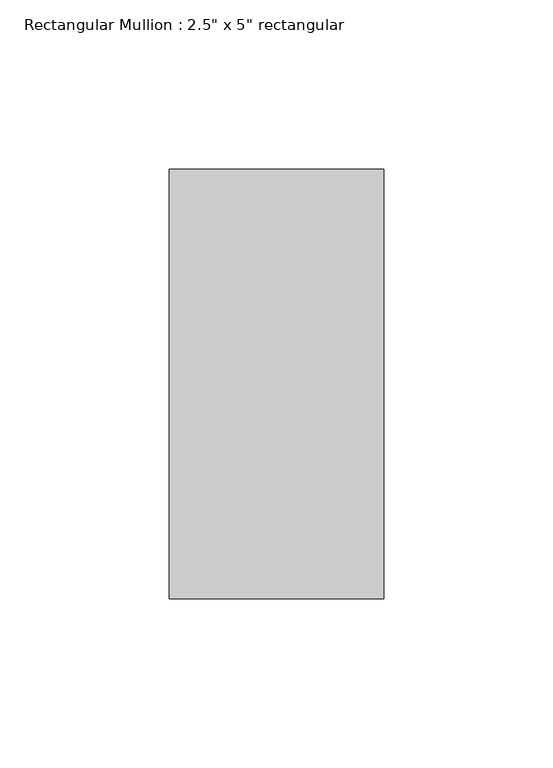
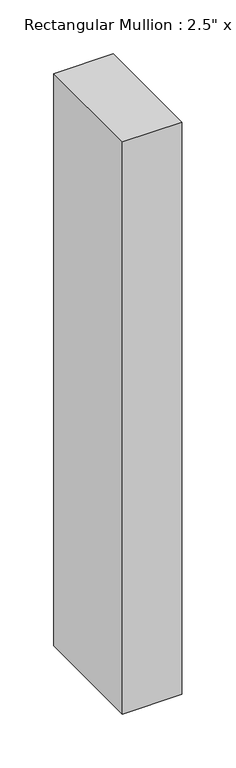
"""IFC4 building model written with IfcOpenShell, lengths in millimetres: member geometry."""

from ifc_helpers import new_model, si_unit, frame, origin, place, context, project, spatial, polyline, outline, extrude, source, transform, mapped, element, save


def member_5215b92c(model_context):
    return source(origin(), model_context, "Body", "SweptSolid", [
        extrude(outline(polyline([(0.0, 63.5), (0.0, -63.5), (-63.5, -63.5), (-63.5, 63.5), (0.0, 63.5)])), frame((0.0, 0.0, -647.7), z_axis=(0.0, 0.0, 1.0), x_axis=(1.0, 0.0, 0.0)), (0.0, 0.0, 1.0), 647.7),
    ])


if __name__ == "__main__":
    model = new_model("IFC4")
    model_context = context("Model", 3, world=origin())
    ifc_project = project(units=[si_unit("LENGTHUNIT", "METRE", prefix="MILLI")], contexts=[model_context])
    site = spatial("IfcSite", under=ifc_project)
    building = spatial("IfcBuilding", under=site)
    placement = place(None, origin())
    member_shape = member_5215b92c(model_context)
    element("IfcMember", 1, ObjectType="Rectangular Mullion : 2.5\" x 5\" rectangular", at=placement, inside=building, context=model_context, shape_type="MappedRepresentation", body=[
        mapped(member_shape, transform((0.0, 0.0, 0.0), x_axis=(1.0, 0.0, 0.0), y_axis=(0.0, 1.0, 0.0), z_axis=(0.0, 0.0, 1.0))),
    ])
    save(model, "model.ifc")

# Revit data of these elements
# Type "Rectangular Mullion : 2.5\" x 5\" rectangular"
#   built-in parameter 1007304 = 0.416667 (stored number, unit not read)
#   built-in parameter 1007301 = 0.104167 (stored number, unit not read)
#   built-in parameter 1007300 = 0.104167 (stored number, unit not read)
# Element 1 (IfcMember, "Rectangular Mullion : 2.5\" x 5\" rectangular")
#   Materials on its faces: "Aluminum"
# Materials
#   "Aluminum": class "Metal", colour RGB 247 247 247, transparency 0, Description = "Aluminum 6061", Cost = 0
